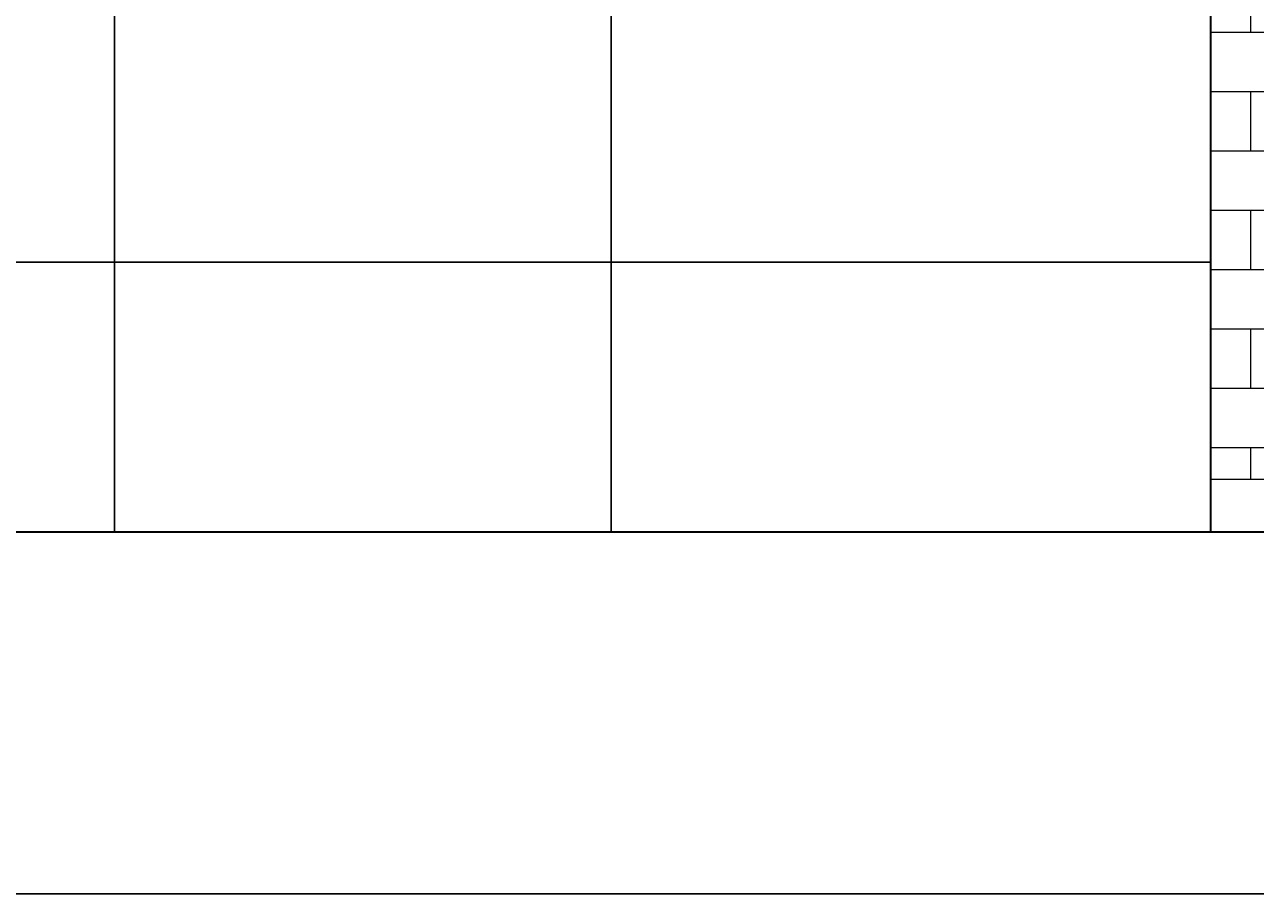
# Model space of a CAD drawing. Units: inches. Extents: x -26 to 776, y -22 to 650.
# Tile 5 of 62: x 98 to 222, y -22 to 67. Entities that reach past the tile are written whole.
import ezdxf

# ---------------------------------------------------------------- set-up
doc = ezdxf.new("R2010")
doc.units = ezdxf.units.IN
doc.header["$MEASUREMENT"] = 0
for name, color, linetype, lineweight in [('A-ANNO-DIMS', 2, 'Continuous', 18), ('A-DOOR', 3, 'Continuous', 25), ('A-WALL-PATT', 8, 'Continuous', 13), ('A-WALL-TRIM', 7, 'Continuous', 18), ('C-TOPO', 7, 'Continuous', 35)]:
    doc.layers.add(name, color=color, linetype=linetype, lineweight=lineweight)
doc.styles.get("Standard").update_dxf_attribs({"font": 'arial.ttf'})
doc.dimstyles.get("Standard").update_dxf_attribs({"dimtxt": 0.5625, "dimasz": 0.18, "dimexe": 0.18, "dimexo": 0.0625, "dimgap": 0.09, "dimtad": 0, "dimtih": 1, "dimtoh": 1, "dimdec": 4, "dimzin": 0, "dimdsep": 46, "dimlunit": 4, "dimtxsty": 'Standard', "dimcen": 0.09, "dimadec": 0, "dimazin": 0, "dimtfac": 1, "dimtdec": 4, "dimtofl": 0, "dimtmove": 0, "dimatfit": 3, "dimfxl": 1, "dimtolj": 1, "dimtzin": 0, "dimarcsym": 0})

# ---------------------------------------------------------------- blocks, each defined once
blk = doc.blocks.new('*D13')
at = {"layer": 'A-ANNO-DIMS', "color": 0, "lineweight": -2, "transparency": 16777216}
for p, q in [((738.75, 50.79), (738.75, -21.31)), ((11.11, 15.42), (11.11, -21.31)), ((11.29, -21.13), (373.89, -21.13)), ((738.57, -21.13), (375.97, -21.13))]:
    blk.add_line(p, q, dxfattribs=at)
at = {"layer": 'A-ANNO-DIMS', "color": 0, "transparency": 16777216}
for points in [[(11.29, -21.1), (11.29, -21.16), (11.11, -21.13)], [(738.57, -21.1), (738.57, -21.16), (738.75, -21.13)]]:
    blk.add_solid(points, dxfattribs=at)
at = {"layer": 'Defpoints', "color": 0, "transparency": 16777216}
for p in [(738.75, 50.85), (11.11, 15.48), (738.75, -21.13)]:
    blk.add_point(p, dxfattribs=at)
at = {"layer": 'A-ANNO-DIMS', "color": 0, "transparency": 16777216, "insert": (374.93, -21.13), "char_height": 0.562, "attachment_point": 5}
blk.add_mtext('\\A1;727.6', dxfattribs=at)
blk = doc.blocks.new('*D14')
at = {"layer": 'A-ANNO-DIMS', "color": 0, "lineweight": -2, "transparency": 16777216}
for p, q in [((191.62, 613.27), (-25.48, 613.27)), ((-25.3, 613.09), (-25.3, 314.75)), ((-25.3, 15.66), (-25.3, 314)), ((11.04, 15.48), (-25.48, 15.48))]:
    blk.add_line(p, q, dxfattribs=at)
at = {"layer": 'A-ANNO-DIMS', "color": 0, "transparency": 16777216}
for points in [[(-25.33, 613.09), (-25.27, 613.09), (-25.3, 613.27)], [(-25.33, 15.66), (-25.27, 15.66), (-25.3, 15.48)]]:
    blk.add_solid(points, dxfattribs=at)
at = {"layer": 'Defpoints', "color": 0, "transparency": 16777216}
for p in [(-25.3, 613.27), (191.68, 613.27), (11.11, 15.48)]:
    blk.add_point(p, dxfattribs=at)
at = {"layer": 'A-ANNO-DIMS', "color": 0, "transparency": 16777216, "insert": (-25.3, 314.38), "char_height": 0.562, "attachment_point": 5}
blk.add_mtext('\\A1;597.8', dxfattribs=at)
blk = doc.blocks.new('*D22')
at = {"layer": 'A-ANNO-DIMS', "color": 0, "lineweight": -2, "transparency": 16777216}
for p, q in [((22.89, 15.33), (22.89, 649.86)), ((217.95, 15.54), (217.95, 649.86)), ((23.07, 649.68), (119.19, 649.68)), ((217.77, 649.68), (121.65, 649.68))]:
    blk.add_line(p, q, dxfattribs=at)
at = {"layer": 'A-ANNO-DIMS', "color": 0, "transparency": 16777216}
for points in [[(23.07, 649.71), (23.07, 649.65), (22.89, 649.68)], [(217.77, 649.71), (217.77, 649.65), (217.95, 649.68)]]:
    blk.add_solid(points, dxfattribs=at)
at = {"layer": 'Defpoints', "color": 0, "transparency": 16777216}
for p in [(217.95, 649.68), (22.89, 15.27), (217.95, 15.48)]:
    blk.add_point(p, dxfattribs=at)
at = {"layer": 'A-ANNO-DIMS', "color": 0, "transparency": 16777216, "insert": (120.42, 649.68), "char_height": 0.562, "attachment_point": 5}
blk.add_mtext('\\A1;195.06', dxfattribs=at)
blk = doc.blocks.new('*D37')
at = {"layer": 'A-ANNO-DIMS', "color": 0, "lineweight": -2, "transparency": 16777216}
for p, q in [((231.36, 159.48), (-25.48, 159.48)), ((-25.3, 159.3), (-25.3, 87.85)), ((-25.3, 15.66), (-25.3, 87.11)), ((217.89, 15.48), (-25.48, 15.48))]:
    blk.add_line(p, q, dxfattribs=at)
at = {"layer": 'A-ANNO-DIMS', "color": 0, "transparency": 16777216}
for points in [[(-25.33, 159.3), (-25.27, 159.3), (-25.3, 159.48)], [(-25.33, 15.66), (-25.27, 15.66), (-25.3, 15.48)]]:
    blk.add_solid(points, dxfattribs=at)
at = {"layer": 'Defpoints', "color": 0, "transparency": 16777216}
for p in [(-25.3, 159.48), (231.42, 159.48), (217.95, 15.48)]:
    blk.add_point(p, dxfattribs=at)
at = {"layer": 'A-ANNO-DIMS', "color": 0, "transparency": 16777216, "insert": (-25.3, 87.48), "char_height": 0.562, "attachment_point": 5}
blk.add_mtext('\\A1;144', dxfattribs=at)

msp = doc.modelspace()

# ---------------------------------------------------------------- hatches: boundary and pattern name
at = {"layer": 'A-WALL-PATT'}
h = msp.add_hatch(dxfattribs=at)
h.set_pattern_fill('AR-B816', color=256, scale=0.75)
h.paths.add_polyline_path([(82.134, 209.6413), (11.1074, 209.6413), (11.1074, 159.4824), (82.134, 159.4824)])
h.paths.add_polyline_path([(231.4249, 209.6413), (209.091, 209.6413), (209.091, 159.4824), (214.1056, 159.4824), (214.1056, 199.3298), (231.4249, 199.3298)])
h.paths.add_polyline_path([(231.4249, 159.4824), (11.1074, 159.4824), (11.1074, 22.5014), (22.8891, 22.5014), (22.8891, 147.0781), (217.9529, 147.0781), (217.9529, 20.7937), (231.4249, 20.7937)])
h.paths.add_polyline_path([(285.0179, 152.3087), (280.6173, 144.8359), (280.6173, 26.4239), (240.1654, 26.4239), (240.1654, 144.8359), (231.4249, 159.4824), (231.4249, 20.7937), (285.0179, 20.7937)])

# ---------------------------------------------------------------- linework, layer by layer
at = {"layer": 'A-DOOR'}
for p, q in [((217.9529, 147.0781), (217.9529, 15.4824)), ((107.0893, 124.9232), (107.0893, 15.4824)), ((157.3287, 124.9232), (157.3287, 15.4824)), ((22.8891, 42.7535), (217.9529, 42.7535))]:
    msp.add_line(p, q, dxfattribs=at)
at = {"layer": 'A-WALL-TRIM'}
msp.add_line((217.9529, 20.7937), (425.7434, 20.7937), dxfattribs=at)
at = {"layer": 'C-TOPO'}
for p, q in [((92.2983, 15.4824), (214.0443, 15.4824)), ((214.0443, 15.4824), (289.2424, 15.4824))]:
    msp.add_line(p, q, dxfattribs=at)

# ---------------------------------------------------------------- dimensions: what is measured, and where the dimension line sits
at = {"layer": 'A-ANNO-DIMS'}
for base, p1, p2, override, picture, middle in [((217.9529, 649.6763), (22.8891, 15.2701), (217.9529, 15.4824), {"dimdec": 2, "dimlfac": 1, "dimrnd": 0, "dimzin": 0, "dimdsep": 46, "dimlunit": 2}, '*D22', (120.421, 649.6763)), ((738.7503, -21.1349), (11.1074, 15.4824), (738.7503, 50.8482), {"dimdec": 1, "dimlfac": 1, "dimrnd": 0, "dimzin": 0, "dimdsep": 46, "dimlunit": 2}, '*D13', (374.9289, -21.1349))]:
    dim = msp.add_linear_dim(base=base, p1=p1, p2=p2, dimstyle='Standard', override=override, dxfattribs=at)
    dim.commit()
    dim.dimension.update_dxf_attribs({"geometry": picture, "text_midpoint": middle})
for base, p1, p2, override, picture, middle in [((-25.2976, 613.2713), (11.1074, 15.4824), (191.6782, 613.2713), {"dimdec": 1, "dimlfac": 1, "dimrnd": 0, "dimzin": 0, "dimdsep": 46, "dimlunit": 2}, '*D14', (-25.2976, 314.3769)), ((-25.2976, 159.4824), (217.9529, 15.4824), (231.4249, 159.4824), {"dimdec": 0, "dimlfac": 1, "dimrnd": 0, "dimzin": 0, "dimdsep": 46, "dimlunit": 2}, '*D37', (-25.2976, 87.4824))]:
    dim = msp.add_linear_dim(base=base, p1=p1, p2=p2, angle=90, dimstyle='Standard', override=override, dxfattribs=at)
    dim.commit()
    dim.dimension.update_dxf_attribs({"geometry": picture, "text_midpoint": middle})

doc.saveas('drawing.dxf')
